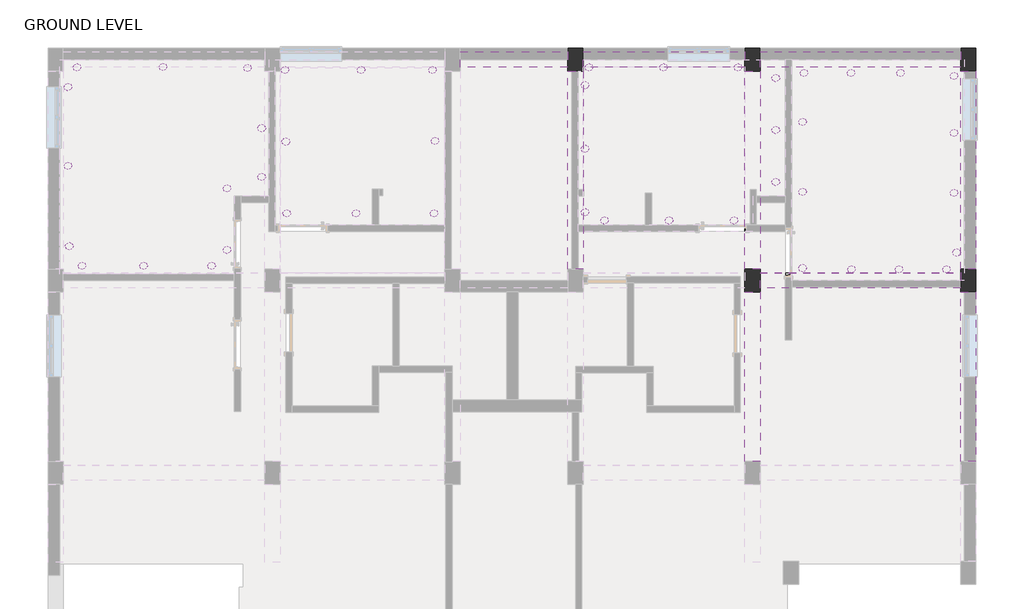
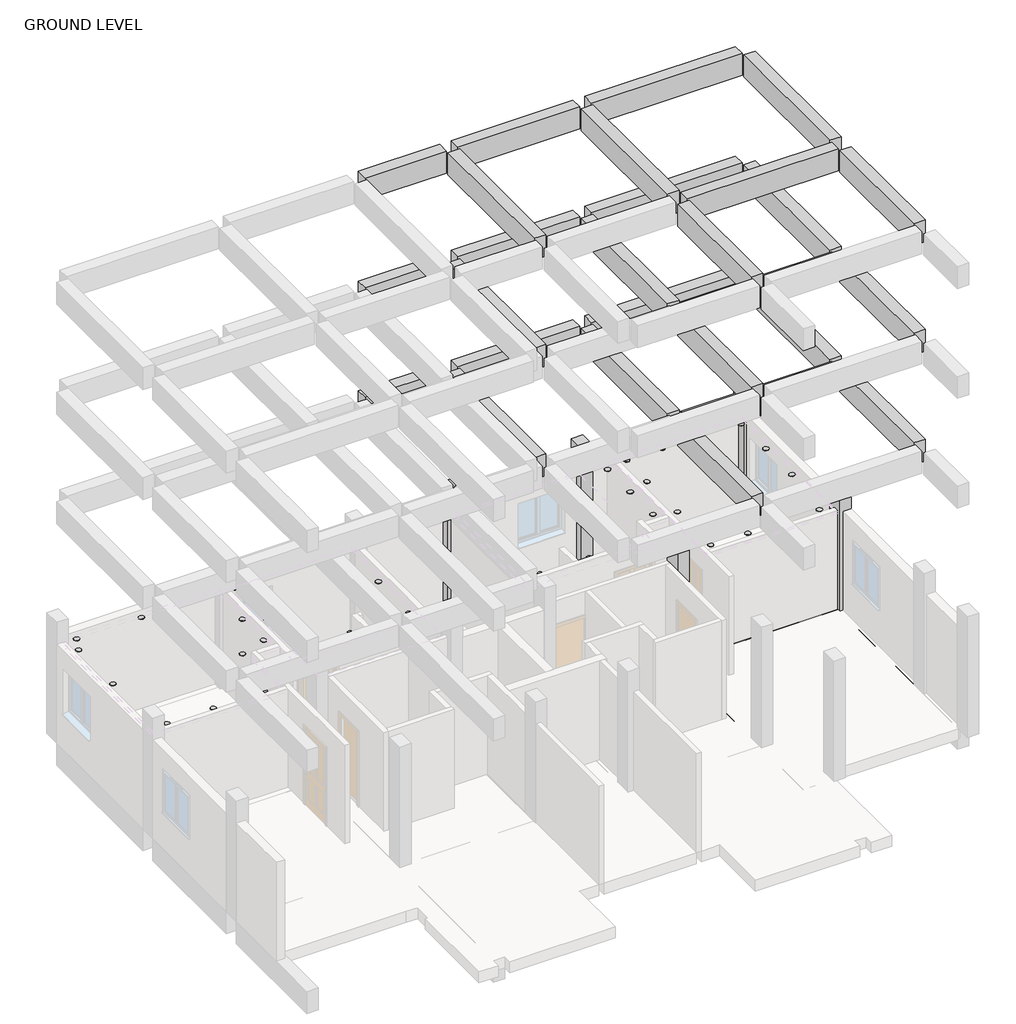
# One storey, part 5 of 5: 46 light fixtures, 36 beams, 5 columns.
"""IFC4 building model written with IfcOpenShell, lengths in millimetres."""

from ifc_helpers import new_model, si_unit, frame, origin, origin_with_axes, place, context, project, spatial, polyline, outline, extrude, faceted_brep, transform, mapped, element, save
from components import family2_family2_8c2629c1

model = new_model("IFC4")

# Units and contexts
model_context = context("Model", 3, world=origin())
ifc_project = project(units=[si_unit("LENGTHUNIT", "METRE", prefix="MILLI")], contexts=[model_context])

# Site, building, storey
site = spatial("IfcSite", under=ifc_project)
building = spatial("IfcBuilding", under=site)
storey = spatial("IfcBuildingStorey", under=building, Name="GROUND LEVEL", Elevation=0.0)

# Beams
placement = place(None, origin())
element("IfcBeam", 1, ObjectType="Concrete-Rectangular Beam : 12 x 24", at=placement, inside=storey, context=model_context, shape_type="SweptSolid", body=[
    extrude(outline(polyline([(1141.4824202, -1299.8061634), (1141.4824202, -1604.6061634), (-992.1175798, -1604.6061634), (-992.1175798, -1299.8061634), (1141.4824202, -1299.8061634)])), frame((0.0, 0.0, -609.6), z_axis=(0.0, 0.0, 1.0), x_axis=(1.0, 0.0, 0.0)), (0.0, 0.0, 1.0), 609.6),
])
element("IfcBeam", 2, ObjectType="Concrete-Rectangular Beam : 12 x 24", at=placement, inside=storey, context=model_context, shape_type="SweptSolid", body=[
    extrude(outline(polyline([(4646.6824202, -1299.8061634), (4646.6824202, -1604.6061634), (1446.2824202, -1604.6061634), (1446.2824202, -1299.8061634), (4646.6824202, -1299.8061634)])), frame((0.0, 0.0, -609.6), z_axis=(0.0, 0.0, 1.0), x_axis=(1.0, 0.0, 0.0)), (0.0, 0.0, 1.0), 609.6),
])
element("IfcBeam", 3, ObjectType="Concrete-Rectangular Beam : 12 x 24", at=placement, inside=storey, context=model_context, shape_type="SweptSolid", body=[
    extrude(outline(polyline([(8913.9345022, -1299.8061634), (8913.9345022, -1604.6061634), (4951.5345022, -1604.6061634), (4951.5345022, -1299.8061634), (8913.9345022, -1299.8061634)])), frame((0.0, 0.0, -609.6), z_axis=(0.0, 0.0, 1.0), x_axis=(1.0, 0.0, 0.0)), (0.0, 0.0, 1.0), 609.6),
])
element("IfcBeam", 4, ObjectType="Concrete-Rectangular Beam : 12 x 24", at=placement, inside=storey, context=model_context, shape_type="SweptSolid", body=[
    extrude(outline(polyline([(9218.6824202, -5600.6620333), (8913.8824202, -5600.6620333), (8913.8824202, -1680.8061634), (9218.6824202, -1680.8061634), (9218.6824202, -5600.6620333)])), frame((0.0, 0.0, -609.6), z_axis=(0.0, 0.0, 1.0), x_axis=(1.0, 0.0, 0.0)), (0.0, 0.0, 1.0), 609.6),
])
element("IfcBeam", 5, ObjectType="Concrete-Rectangular Beam : 12 x 24", at=placement, inside=storey, context=model_context, shape_type="SweptSolid", body=[
    extrude(outline(polyline([(9218.6824202, -9410.6620333), (8913.8824202, -9410.6620333), (8913.8824202, -6057.8620333), (9218.6824202, -6057.8620333), (9218.6824202, -9410.6620333)])), frame((0.0, 0.0, -609.6), z_axis=(0.0, 0.0, 1.0), x_axis=(1.0, 0.0, 0.0)), (0.0, 0.0, 1.0), 609.6),
])
element("IfcBeam", 6, ObjectType="Concrete-Rectangular Beam : 12 x 24", at=placement, inside=storey, context=model_context, shape_type="SweptSolid", body=[
    extrude(outline(polyline([(4951.4824202, -5981.6620333), (4951.4824202, -5676.8620333), (8913.8824202, -5676.8620333), (8913.8824202, -5981.6620333), (4951.4824202, -5981.6620333)])), frame((0.0, 0.0, -609.6), z_axis=(0.0, 0.0, 1.0), x_axis=(1.0, 0.0, 0.0)), (0.0, 0.0, 1.0), 609.6),
])
element("IfcBeam", 7, ObjectType="Concrete-Rectangular Beam : 12 x 24", at=placement, inside=storey, context=model_context, shape_type="SweptSolid", body=[
    extrude(outline(polyline([(1141.4824202, -1680.8061634), (1446.2824202, -1680.8061634), (1446.2824202, -5600.6620333), (1141.4824202, -5600.6620333), (1141.4824202, -1680.8061634)])), frame((0.0, 0.0, -609.6), z_axis=(0.0, 0.0, 1.0), x_axis=(1.0, 0.0, 0.0)), (0.0, 0.0, 1.0), 609.6),
])
element("IfcBeam", 8, ObjectType="Concrete-Rectangular Beam : 12 x 24", at=placement, inside=storey, context=model_context, shape_type="SweptSolid", body=[
    extrude(outline(polyline([(4951.4824202, -5600.6620333), (4646.6824202, -5600.6620333), (4646.6824202, -1680.8061634), (4951.4824202, -1680.8061634), (4951.4824202, -5600.6620333)])), frame((0.0, 0.0, -609.6), z_axis=(0.0, 0.0, 1.0), x_axis=(1.0, 0.0, 0.0)), (0.0, 0.0, 1.0), 609.6),
])
element("IfcBeam", 9, ObjectType="Concrete-Rectangular Beam : 12 x 24", at=placement, inside=storey, context=model_context, shape_type="SweptSolid", body=[
    extrude(outline(polyline([(4951.4824202, -9410.6620333), (4646.6824202, -9410.6620333), (4646.6824202, -6057.8620333), (4951.4824202, -6057.8620333), (4951.4824202, -9410.6620333)])), frame((0.0, 0.0, -609.6), z_axis=(0.0, 0.0, 1.0), x_axis=(1.0, 0.0, 0.0)), (0.0, 0.0, 1.0), 609.6),
])
element("IfcBeam", 10, ObjectType="Concrete-Rectangular Beam : 12 x 24", at=placement, inside=storey, context=model_context, shape_type="SweptSolid", body=[
    extrude(outline(polyline([(1141.4824202, -1299.8061634), (1141.4824202, -1604.6061634), (-992.1175798, -1604.6061634), (-992.1175798, -1299.8061634), (1141.4824202, -1299.8061634)])), frame((0.0, 0.0, 6096.0), z_axis=(0.0, 0.0, 1.0), x_axis=(1.0, 0.0, 0.0)), (0.0, 0.0, 1.0), 609.6),
])
element("IfcBeam", 11, ObjectType="Concrete-Rectangular Beam : 12 x 24", at=placement, inside=storey, context=model_context, shape_type="SweptSolid", body=[
    extrude(outline(polyline([(4646.6824202, -1299.8061634), (4646.6824202, -1604.6061634), (1446.2824202, -1604.6061634), (1446.2824202, -1299.8061634), (4646.6824202, -1299.8061634)])), frame((0.0, 0.0, 6096.0), z_axis=(0.0, 0.0, 1.0), x_axis=(1.0, 0.0, 0.0)), (0.0, 0.0, 1.0), 609.6),
])
element("IfcBeam", 12, ObjectType="Concrete-Rectangular Beam : 12 x 24", at=placement, inside=storey, context=model_context, shape_type="SweptSolid", body=[
    extrude(outline(polyline([(8913.9345022, -1299.8061634), (8913.9345022, -1604.6061634), (4951.5345022, -1604.6061634), (4951.5345022, -1299.8061634), (8913.9345022, -1299.8061634)])), frame((0.0, 0.0, 6096.0), z_axis=(0.0, 0.0, 1.0), x_axis=(1.0, 0.0, 0.0)), (0.0, 0.0, 1.0), 609.6),
])
element("IfcBeam", 13, ObjectType="Concrete-Rectangular Beam : 12 x 24", at=placement, inside=storey, context=model_context, shape_type="Brep", body=[
    faceted_brep([(8913.8824202, -5600.6620333, 6705.6), (9218.6824202, -5600.6620333, 6705.6), (9218.6824202, -1680.8061634, 6705.6), (8913.8824202, -1680.8061634, 6705.6), (8913.8824202, -5600.6620333, 6096.0), (8913.8824202, -5600.6620333, 6400.8), (8913.8824202, -1680.8061634, 6400.8), (8913.8824202, -1680.8061634, 6096.0), (9218.6824202, -5600.6620333, 6096.0), (9218.6824202, -1680.8061634, 6096.0), (9218.6824202, -5600.6620333, 6400.8), (9218.6824202, -1680.8061634, 6400.8)], [[[0, 1, 2, 3]], [[4, 5, 0, 3, 6, 7]], [[8, 4, 7, 9]], [[1, 10, 8, 9, 11, 2]], [[2, 11, 9, 7, 6, 3]], [[1, 0, 5, 4, 8, 10]]]),
])
element("IfcBeam", 14, ObjectType="Concrete-Rectangular Beam : 12 x 24", at=placement, inside=storey, context=model_context, shape_type="Brep", body=[
    faceted_brep([(8913.8824202, -9410.6620333, 6705.6), (9218.6824202, -9410.6620333, 6705.6), (9218.6824202, -6057.8620333, 6705.6), (8913.8824202, -6057.8620333, 6705.6), (8913.8824202, -9410.6620333, 6096.0), (8913.8824202, -9410.6620333, 6400.8), (8913.8824202, -6057.8620333, 6400.8), (8913.8824202, -6057.8620333, 6096.0), (9218.6824202, -9410.6620333, 6096.0), (9218.6824202, -6057.8620333, 6096.0), (9218.6824202, -9410.6620333, 6400.8), (9218.6824202, -6057.8620333, 6400.8)], [[[0, 1, 2, 3]], [[4, 5, 0, 3, 6, 7]], [[8, 4, 7, 9]], [[1, 10, 8, 9, 11, 2]], [[2, 11, 9, 7, 6, 3]], [[1, 0, 5, 4, 8, 10]]]),
])
element("IfcBeam", 15, ObjectType="Concrete-Rectangular Beam : 12 x 24", at=placement, inside=storey, context=model_context, shape_type="SweptSolid", body=[
    extrude(outline(polyline([(4951.4824202, -5981.6620333), (4951.4824202, -5676.8620333), (8913.8824202, -5676.8620333), (8913.8824202, -5981.6620333), (4951.4824202, -5981.6620333)])), frame((0.0, 0.0, 6096.0), z_axis=(0.0, 0.0, 1.0), x_axis=(1.0, 0.0, 0.0)), (0.0, 0.0, 1.0), 609.6),
])
element("IfcBeam", 16, ObjectType="Concrete-Rectangular Beam : 12 x 24", at=placement, inside=storey, context=model_context, shape_type="Brep", body=[
    faceted_brep([(1446.2824202, -1680.8061634, 6705.6), (1141.4824202, -1680.8061634, 6705.6), (1141.4824202, -5600.6620333, 6705.6), (1446.2824202, -5600.6620333, 6705.6), (1446.2824202, -1680.8061634, 6096.0), (1446.2824202, -1680.8061634, 6400.8), (1446.2824202, -5600.6620333, 6400.8), (1446.2824202, -5600.6620333, 6096.0), (1141.4824202, -1680.8061634, 6096.0), (1141.4824202, -5600.6620333, 6096.0), (1141.4824202, -1680.8061634, 6400.8), (1141.4824202, -5600.6620333, 6400.8)], [[[0, 1, 2, 3]], [[4, 5, 0, 3, 6, 7]], [[8, 4, 7, 9]], [[1, 10, 8, 9, 11, 2]], [[1, 0, 5, 4, 8, 10]], [[2, 11, 9, 7, 6, 3]]]),
])
element("IfcBeam", 17, ObjectType="Concrete-Rectangular Beam : 12 x 24", at=placement, inside=storey, context=model_context, shape_type="Brep", body=[
    faceted_brep([(4646.6824202, -5600.6620333, 6705.6), (4951.4824202, -5600.6620333, 6705.6), (4951.4824202, -1680.8061634, 6705.6), (4646.6824202, -1680.8061634, 6705.6), (4646.6824202, -5600.6620333, 6096.0), (4646.6824202, -5600.6620333, 6400.8), (4646.6824202, -1680.8061634, 6400.8), (4646.6824202, -1680.8061634, 6096.0), (4951.4824202, -5600.6620333, 6096.0), (4951.4824202, -1680.8061634, 6096.0), (4951.4824202, -5600.6620333, 6400.8), (4951.4824202, -1680.8061634, 6400.8)], [[[0, 1, 2, 3]], [[4, 5, 0, 3, 6, 7]], [[8, 4, 7, 9]], [[1, 10, 8, 9, 11, 2]], [[2, 11, 9, 7, 6, 3]], [[1, 0, 5, 4, 8, 10]]]),
])
element("IfcBeam", 18, ObjectType="Concrete-Rectangular Beam : 12 x 24", at=placement, inside=storey, context=model_context, shape_type="Brep", body=[
    faceted_brep([(4646.6824202, -9410.6620333, 6705.6), (4951.4824202, -9410.6620333, 6705.6), (4951.4824202, -6057.8620333, 6705.6), (4646.6824202, -6057.8620333, 6705.6), (4646.6824202, -9410.6620333, 6096.0), (4646.6824202, -9410.6620333, 6400.8), (4646.6824202, -6057.8620333, 6400.8), (4646.6824202, -6057.8620333, 6096.0), (4951.4824202, -9410.6620333, 6096.0), (4951.4824202, -6057.8620333, 6096.0), (4951.4824202, -9410.6620333, 6400.8), (4951.4824202, -6057.8620333, 6400.8)], [[[0, 1, 2, 3]], [[4, 5, 0, 3, 6, 7]], [[8, 4, 7, 9]], [[1, 10, 8, 9, 11, 2]], [[2, 11, 9, 7, 6, 3]], [[1, 0, 5, 4, 8, 10]]]),
])
element("IfcBeam", 19, ObjectType="Concrete-Rectangular Beam : 12 x 24", at=placement, inside=storey, context=model_context, shape_type="SweptSolid", body=[
    extrude(outline(polyline([(1141.4824202, -1299.8061634), (1141.4824202, -1604.6061634), (-992.1175798, -1604.6061634), (-992.1175798, -1299.8061634), (1141.4824202, -1299.8061634)])), frame((0.0, 0.0, 9144.0), z_axis=(0.0, 0.0, 1.0), x_axis=(1.0, 0.0, 0.0)), (0.0, 0.0, 1.0), 609.6),
])
element("IfcBeam", 20, ObjectType="Concrete-Rectangular Beam : 12 x 24", at=placement, inside=storey, context=model_context, shape_type="SweptSolid", body=[
    extrude(outline(polyline([(4646.6824202, -1299.8061634), (4646.6824202, -1604.6061634), (1446.2824202, -1604.6061634), (1446.2824202, -1299.8061634), (4646.6824202, -1299.8061634)])), frame((0.0, 0.0, 9144.0), z_axis=(0.0, 0.0, 1.0), x_axis=(1.0, 0.0, 0.0)), (0.0, 0.0, 1.0), 609.6),
])
element("IfcBeam", 21, ObjectType="Concrete-Rectangular Beam : 12 x 24", at=placement, inside=storey, context=model_context, shape_type="SweptSolid", body=[
    extrude(outline(polyline([(8913.9345022, -1299.8061634), (8913.9345022, -1604.6061634), (4951.5345022, -1604.6061634), (4951.5345022, -1299.8061634), (8913.9345022, -1299.8061634)])), frame((0.0, 0.0, 9144.0), z_axis=(0.0, 0.0, 1.0), x_axis=(1.0, 0.0, 0.0)), (0.0, 0.0, 1.0), 609.6),
])
element("IfcBeam", 22, ObjectType="Concrete-Rectangular Beam : 12 x 24", at=placement, inside=storey, context=model_context, shape_type="Brep", body=[
    faceted_brep([(8913.8824202, -5600.6620333, 9753.6), (9218.6824202, -5600.6620333, 9753.6), (9218.6824202, -1680.8061634, 9753.6), (8913.8824202, -1680.8061634, 9753.6), (8913.8824202, -5600.6620333, 9144.0), (8913.8824202, -5600.6620333, 9448.8), (8913.8824202, -1680.8061634, 9448.8), (8913.8824202, -1680.8061634, 9144.0), (9218.6824202, -5600.6620333, 9144.0), (9218.6824202, -1680.8061634, 9144.0), (9218.6824202, -5600.6620333, 9448.8), (9218.6824202, -1680.8061634, 9448.8)], [[[0, 1, 2, 3]], [[4, 5, 0, 3, 6, 7]], [[8, 4, 7, 9]], [[1, 10, 8, 9, 11, 2]], [[2, 11, 9, 7, 6, 3]], [[1, 0, 5, 4, 8, 10]]]),
])
element("IfcBeam", 23, ObjectType="Concrete-Rectangular Beam : 12 x 24", at=placement, inside=storey, context=model_context, shape_type="Brep", body=[
    faceted_brep([(8913.8824202, -9410.6620333, 9753.6), (9218.6824202, -9410.6620333, 9753.6), (9218.6824202, -6057.8620333, 9753.6), (8913.8824202, -6057.8620333, 9753.6), (8913.8824202, -9410.6620333, 9144.0), (8913.8824202, -9410.6620333, 9448.8), (8913.8824202, -6057.8620333, 9448.8), (8913.8824202, -6057.8620333, 9144.0), (9218.6824202, -9410.6620333, 9144.0), (9218.6824202, -6057.8620333, 9144.0), (9218.6824202, -9410.6620333, 9448.8), (9218.6824202, -6057.8620333, 9448.8)], [[[0, 1, 2, 3]], [[4, 5, 0, 3, 6, 7]], [[8, 4, 7, 9]], [[1, 10, 8, 9, 11, 2]], [[2, 11, 9, 7, 6, 3]], [[1, 0, 5, 4, 8, 10]]]),
])
element("IfcBeam", 24, ObjectType="Concrete-Rectangular Beam : 12 x 24", at=placement, inside=storey, context=model_context, shape_type="SweptSolid", body=[
    extrude(outline(polyline([(4951.4824202, -5981.6620333), (4951.4824202, -5676.8620333), (8913.8824202, -5676.8620333), (8913.8824202, -5981.6620333), (4951.4824202, -5981.6620333)])), frame((0.0, 0.0, 9144.0), z_axis=(0.0, 0.0, 1.0), x_axis=(1.0, 0.0, 0.0)), (0.0, 0.0, 1.0), 609.6),
])
element("IfcBeam", 25, ObjectType="Concrete-Rectangular Beam : 12 x 24", at=placement, inside=storey, context=model_context, shape_type="Brep", body=[
    faceted_brep([(1446.2824202, -1680.8061634, 9753.6), (1141.4824202, -1680.8061634, 9753.6), (1141.4824202, -5600.6620333, 9753.6), (1446.2824202, -5600.6620333, 9753.6), (1446.2824202, -1680.8061634, 9144.0), (1446.2824202, -1680.8061634, 9448.8), (1446.2824202, -5600.6620333, 9448.8), (1446.2824202, -5600.6620333, 9144.0), (1141.4824202, -1680.8061634, 9144.0), (1141.4824202, -5600.6620333, 9144.0), (1141.4824202, -1680.8061634, 9448.8), (1141.4824202, -5600.6620333, 9448.8)], [[[0, 1, 2, 3]], [[4, 5, 0, 3, 6, 7]], [[8, 4, 7, 9]], [[1, 10, 8, 9, 11, 2]], [[1, 0, 5, 4, 8, 10]], [[2, 11, 9, 7, 6, 3]]]),
])
element("IfcBeam", 26, ObjectType="Concrete-Rectangular Beam : 12 x 24", at=placement, inside=storey, context=model_context, shape_type="Brep", body=[
    faceted_brep([(4646.6824202, -5600.6620333, 9753.6), (4951.4824202, -5600.6620333, 9753.6), (4951.4824202, -1680.8061634, 9753.6), (4646.6824202, -1680.8061634, 9753.6), (4646.6824202, -5600.6620333, 9144.0), (4646.6824202, -5600.6620333, 9448.8), (4646.6824202, -1680.8061634, 9448.8), (4646.6824202, -1680.8061634, 9144.0), (4951.4824202, -5600.6620333, 9144.0), (4951.4824202, -1680.8061634, 9144.0), (4951.4824202, -5600.6620333, 9448.8), (4951.4824202, -1680.8061634, 9448.8)], [[[0, 1, 2, 3]], [[4, 5, 0, 3, 6, 7]], [[8, 4, 7, 9]], [[1, 10, 8, 9, 11, 2]], [[2, 11, 9, 7, 6, 3]], [[1, 0, 5, 4, 8, 10]]]),
])
element("IfcBeam", 27, ObjectType="Concrete-Rectangular Beam : 12 x 24", at=placement, inside=storey, context=model_context, shape_type="Brep", body=[
    faceted_brep([(4646.6824202, -9410.6620333, 9753.6), (4951.4824202, -9410.6620333, 9753.6), (4951.4824202, -6057.8620333, 9753.6), (4646.6824202, -6057.8620333, 9753.6), (4646.6824202, -9410.6620333, 9144.0), (4646.6824202, -9410.6620333, 9448.8), (4646.6824202, -6057.8620333, 9448.8), (4646.6824202, -6057.8620333, 9144.0), (4951.4824202, -9410.6620333, 9144.0), (4951.4824202, -6057.8620333, 9144.0), (4951.4824202, -9410.6620333, 9448.8), (4951.4824202, -6057.8620333, 9448.8)], [[[0, 1, 2, 3]], [[4, 5, 0, 3, 6, 7]], [[8, 4, 7, 9]], [[1, 10, 8, 9, 11, 2]], [[2, 11, 9, 7, 6, 3]], [[1, 0, 5, 4, 8, 10]]]),
])
element("IfcBeam", 28, ObjectType="Concrete-Rectangular Beam : 12 x 24", at=placement, inside=storey, context=model_context, shape_type="SweptSolid", body=[
    extrude(outline(polyline([(1141.4824202, -1299.8061634), (1141.4824202, -1604.6061634), (-992.1175798, -1604.6061634), (-992.1175798, -1299.8061634), (1141.4824202, -1299.8061634)])), frame((0.0, 0.0, 12192.0), z_axis=(0.0, 0.0, 1.0), x_axis=(1.0, 0.0, 0.0)), (0.0, 0.0, 1.0), 609.6),
])
element("IfcBeam", 29, ObjectType="Concrete-Rectangular Beam : 12 x 24", at=placement, inside=storey, context=model_context, shape_type="SweptSolid", body=[
    extrude(outline(polyline([(4646.6824202, -1299.8061634), (4646.6824202, -1604.6061634), (1446.2824202, -1604.6061634), (1446.2824202, -1299.8061634), (4646.6824202, -1299.8061634)])), frame((0.0, 0.0, 12192.0), z_axis=(0.0, 0.0, 1.0), x_axis=(1.0, 0.0, 0.0)), (0.0, 0.0, 1.0), 609.6),
])
element("IfcBeam", 30, ObjectType="Concrete-Rectangular Beam : 12 x 24", at=placement, inside=storey, context=model_context, shape_type="SweptSolid", body=[
    extrude(outline(polyline([(8913.9345022, -1299.8061634), (8913.9345022, -1604.6061634), (4951.5345022, -1604.6061634), (4951.5345022, -1299.8061634), (8913.9345022, -1299.8061634)])), frame((0.0, 0.0, 12192.0), z_axis=(0.0, 0.0, 1.0), x_axis=(1.0, 0.0, 0.0)), (0.0, 0.0, 1.0), 609.6),
])
element("IfcBeam", 31, ObjectType="Concrete-Rectangular Beam : 12 x 24", at=placement, inside=storey, context=model_context, shape_type="SweptSolid", body=[
    extrude(outline(polyline([(9218.6824202, -5600.6620333), (8913.8824202, -5600.6620333), (8913.8824202, -1680.8061634), (9218.6824202, -1680.8061634), (9218.6824202, -5600.6620333)])), frame((0.0, 0.0, 12192.0), z_axis=(0.0, 0.0, 1.0), x_axis=(1.0, 0.0, 0.0)), (0.0, 0.0, 1.0), 609.6),
])
element("IfcBeam", 32, ObjectType="Concrete-Rectangular Beam : 12 x 24", at=placement, inside=storey, context=model_context, shape_type="SweptSolid", body=[
    extrude(outline(polyline([(9218.6824202, -9410.6620333), (8913.8824202, -9410.6620333), (8913.8824202, -6057.8620333), (9218.6824202, -6057.8620333), (9218.6824202, -9410.6620333)])), frame((0.0, 0.0, 12192.0), z_axis=(0.0, 0.0, 1.0), x_axis=(1.0, 0.0, 0.0)), (0.0, 0.0, 1.0), 609.6),
])
element("IfcBeam", 33, ObjectType="Concrete-Rectangular Beam : 12 x 24", at=placement, inside=storey, context=model_context, shape_type="SweptSolid", body=[
    extrude(outline(polyline([(4951.4824202, -5981.6620333), (4951.4824202, -5676.8620333), (8913.8824202, -5676.8620333), (8913.8824202, -5981.6620333), (4951.4824202, -5981.6620333)])), frame((0.0, 0.0, 12192.0), z_axis=(0.0, 0.0, 1.0), x_axis=(1.0, 0.0, 0.0)), (0.0, 0.0, 1.0), 609.6),
])
element("IfcBeam", 34, ObjectType="Concrete-Rectangular Beam : 12 x 24", at=placement, inside=storey, context=model_context, shape_type="SweptSolid", body=[
    extrude(outline(polyline([(1141.4824202, -1680.8061634), (1446.2824202, -1680.8061634), (1446.2824202, -5600.6620333), (1141.4824202, -5600.6620333), (1141.4824202, -1680.8061634)])), frame((0.0, 0.0, 12192.0), z_axis=(0.0, 0.0, 1.0), x_axis=(1.0, 0.0, 0.0)), (0.0, 0.0, 1.0), 609.6),
])
element("IfcBeam", 35, ObjectType="Concrete-Rectangular Beam : 12 x 24", at=placement, inside=storey, context=model_context, shape_type="SweptSolid", body=[
    extrude(outline(polyline([(4951.4824202, -5600.6620333), (4646.6824202, -5600.6620333), (4646.6824202, -1680.8061634), (4951.4824202, -1680.8061634), (4951.4824202, -5600.6620333)])), frame((0.0, 0.0, 12192.0), z_axis=(0.0, 0.0, 1.0), x_axis=(1.0, 0.0, 0.0)), (0.0, 0.0, 1.0), 609.6),
])
element("IfcBeam", 36, ObjectType="Concrete-Rectangular Beam : 12 x 24", at=placement, inside=storey, context=model_context, shape_type="SweptSolid", body=[
    extrude(outline(polyline([(4951.4824202, -9410.6620333), (4646.6824202, -9410.6620333), (4646.6824202, -6057.8620333), (4951.4824202, -6057.8620333), (4951.4824202, -9410.6620333)])), frame((0.0, 0.0, 12192.0), z_axis=(0.0, 0.0, 1.0), x_axis=(1.0, 0.0, 0.0)), (0.0, 0.0, 1.0), 609.6),
])

# Columns
element("IfcColumn", 37, ObjectType="Concrete-Rectangular-Column : 1'6\" X 1' COLUMN", at=placement, inside=storey, context=model_context, shape_type="SweptSolid", body=[
    extrude(outline(polyline([(1446.2824202, -1223.6061634), (1446.2824202, -1680.8061634), (1141.4824202, -1680.8061634), (1141.4824202, -1223.6061634), (1446.2824202, -1223.6061634)])), origin_with_axes(), (0.0, 0.0, 1.0), 3352.8),
])
element("IfcColumn", 38, ObjectType="Concrete-Rectangular-Column : 1'6\" X 1' COLUMN", at=placement, inside=storey, context=model_context, shape_type="SweptSolid", body=[
    extrude(outline(polyline([(4951.4824202, -1223.6061634), (4951.4824202, -1680.8061634), (4646.6824202, -1680.8061634), (4646.6824202, -1223.6061634), (4951.4824202, -1223.6061634)])), origin_with_axes(), (0.0, 0.0, 1.0), 3352.8),
])
element("IfcColumn", 39, ObjectType="Concrete-Rectangular-Column : 1'6\" X 1' COLUMN", at=placement, inside=storey, context=model_context, shape_type="SweptSolid", body=[
    extrude(outline(polyline([(9218.6824202, -1223.6061634), (9218.6824202, -1680.8061634), (8913.8824202, -1680.8061634), (8913.8824202, -1223.6061634), (9218.6824202, -1223.6061634)])), origin_with_axes(), (0.0, 0.0, 1.0), 3352.8),
])
element("IfcColumn", 40, ObjectType="Concrete-Rectangular-Column : 1'6\" X 1' COLUMN", at=placement, inside=storey, context=model_context, shape_type="SweptSolid", body=[
    extrude(outline(polyline([(9218.6824202, -5600.6620333), (9218.6824202, -6057.8620333), (8913.8824202, -6057.8620333), (8913.8824202, -5600.6620333), (9218.6824202, -5600.6620333)])), origin_with_axes(), (0.0, 0.0, 1.0), 3352.8),
])
element("IfcColumn", 41, ObjectType="Concrete-Rectangular-Column : 1'6\" X 1' COLUMN", at=placement, inside=storey, context=model_context, shape_type="SweptSolid", body=[
    extrude(outline(polyline([(4951.4824202, -5600.6620333), (4951.4824202, -6057.8620333), (4646.6824202, -6057.8620333), (4646.6824202, -5600.6620333), (4951.4824202, -5600.6620333)])), origin_with_axes(), (0.0, 0.0, 1.0), 3352.8),
])

# Light fixtures
family2_family2_shape = family2_family2_8c2629c1(model_context)
element("IfcLightFixture", 42, ObjectType="Family2 : Family2", at=placement, inside=storey, context=model_context, shape_type="MappedRepresentation", body=[
    mapped(family2_family2_shape, transform((-4916.4175798, -3776.3061634, 101.6), x_axis=(1.0, 0.0, 0.0), y_axis=(0.0, 1.0, 0.0), z_axis=(0.0, 0.0, 1.0))),
])
element("IfcLightFixture", 43, ObjectType="Family2 : Family2", at=placement, inside=storey, context=model_context, shape_type="MappedRepresentation", body=[
    mapped(family2_family2_shape, transform((-4916.4175798, -2811.1061634, 101.6), x_axis=(1.0, 0.0, 0.0), y_axis=(0.0, 1.0, 0.0), z_axis=(0.0, 0.0, 1.0))),
])
element("IfcLightFixture", 44, ObjectType="Family2 : Family2", at=placement, inside=storey, context=model_context, shape_type="MappedRepresentation", body=[
    mapped(family2_family2_shape, transform((-5195.8175798, -1617.3061634, 101.6), x_axis=(1.0, 0.0, 0.0), y_axis=(0.0, 1.0, 0.0), z_axis=(0.0, 0.0, 1.0))),
])
element("IfcLightFixture", 45, ObjectType="Family2 : Family2", at=placement, inside=storey, context=model_context, shape_type="MappedRepresentation", body=[
    mapped(family2_family2_shape, transform((-8573.2786397, -1604.6061634, 101.6), x_axis=(1.0, 0.0, 0.0), y_axis=(0.0, 1.0, 0.0), z_axis=(0.0, 0.0, 1.0))),
])
element("IfcLightFixture", 46, ObjectType="Family2 : Family2", at=placement, inside=storey, context=model_context, shape_type="MappedRepresentation", body=[
    mapped(family2_family2_shape, transform((-6871.4786397, -1598.2561634, 101.6), x_axis=(1.0, 0.0, 0.0), y_axis=(0.0, 1.0, 0.0), z_axis=(0.0, 0.0, 1.0))),
])
element("IfcLightFixture", 47, ObjectType="Family2 : Family2", at=placement, inside=storey, context=model_context, shape_type="MappedRepresentation", body=[
    mapped(family2_family2_shape, transform((-8751.0786397, -1998.3061634, 101.6), x_axis=(1.0, 0.0, 0.0), y_axis=(0.0, 1.0, 0.0), z_axis=(0.0, 0.0, 1.0))),
])
element("IfcLightFixture", 48, ObjectType="Family2 : Family2", at=placement, inside=storey, context=model_context, shape_type="MappedRepresentation", body=[
    mapped(family2_family2_shape, transform((-8725.6786397, -5147.9061634, 101.6), x_axis=(1.0, 0.0, 0.0), y_axis=(0.0, 1.0, 0.0), z_axis=(0.0, 0.0, 1.0))),
])
element("IfcLightFixture", 49, ObjectType="Family2 : Family2", at=placement, inside=storey, context=model_context, shape_type="MappedRepresentation", body=[
    mapped(family2_family2_shape, transform((-8751.0786397, -3556.4104011, 101.6), x_axis=(1.0, 0.0, 0.0), y_axis=(0.0, 1.0, 0.0), z_axis=(0.0, 0.0, 1.0))),
])
element("IfcLightFixture", 50, ObjectType="Family2 : Family2", at=placement, inside=storey, context=model_context, shape_type="MappedRepresentation", body=[
    mapped(family2_family2_shape, transform((-8471.6786397, -5537.1620333, 101.6), x_axis=(1.0, 0.0, 0.0), y_axis=(0.0, 1.0, 0.0), z_axis=(0.0, 0.0, 1.0))),
])
element("IfcLightFixture", 51, ObjectType="Family2 : Family2", at=placement, inside=storey, context=model_context, shape_type="MappedRepresentation", body=[
    mapped(family2_family2_shape, transform((-5907.0175798, -5537.1620333, 101.6), x_axis=(1.0, 0.0, 0.0), y_axis=(0.0, 1.0, 0.0), z_axis=(0.0, 0.0, 1.0))),
])
element("IfcLightFixture", 52, ObjectType="Family2 : Family2", at=placement, inside=storey, context=model_context, shape_type="MappedRepresentation", body=[
    mapped(family2_family2_shape, transform((-7252.4786397, -5537.1620333, 101.6), x_axis=(1.0, 0.0, 0.0), y_axis=(0.0, 1.0, 0.0), z_axis=(0.0, 0.0, 1.0))),
])
element("IfcLightFixture", 53, ObjectType="Family2 : Family2", at=placement, inside=storey, context=model_context, shape_type="MappedRepresentation", body=[
    mapped(family2_family2_shape, transform((-5602.2175798, -5224.1061634, 101.6), x_axis=(1.0, 0.0, 0.0), y_axis=(0.0, 1.0, 0.0), z_axis=(0.0, 0.0, 1.0))),
])
element("IfcLightFixture", 54, ObjectType="Family2 : Family2", at=placement, inside=storey, context=model_context, shape_type="MappedRepresentation", body=[
    mapped(family2_family2_shape, transform((-5602.2175798, -4004.9061634, 101.6), x_axis=(1.0, 0.0, 0.0), y_axis=(0.0, 1.0, 0.0), z_axis=(0.0, 0.0, 1.0))),
])
element("IfcLightFixture", 55, ObjectType="Family2 : Family2", at=placement, inside=storey, context=model_context, shape_type="MappedRepresentation", body=[
    mapped(family2_family2_shape, transform((5815.0824202, -1718.9061634, 101.6), x_axis=(1.0, 0.0, 0.0), y_axis=(0.0, 1.0, 0.0), z_axis=(0.0, 0.0, 1.0))),
])
element("IfcLightFixture", 56, ObjectType="Family2 : Family2", at=placement, inside=storey, context=model_context, shape_type="MappedRepresentation", body=[
    mapped(family2_family2_shape, transform((8786.8824202, -1776.0561634, 101.6), x_axis=(1.0, 0.0, 0.0), y_axis=(0.0, 1.0, 0.0), z_axis=(0.0, 0.0, 1.0))),
])
element("IfcLightFixture", 57, ObjectType="Family2 : Family2", at=placement, inside=storey, context=model_context, shape_type="MappedRepresentation", body=[
    mapped(family2_family2_shape, transform((6746.4157535, -1718.9061634, 101.6), x_axis=(1.0, 0.0, 0.0), y_axis=(0.0, 1.0, 0.0), z_axis=(0.0, 0.0, 1.0))),
])
element("IfcLightFixture", 58, ObjectType="Family2 : Family2", at=placement, inside=storey, context=model_context, shape_type="MappedRepresentation", body=[
    mapped(family2_family2_shape, transform((7728.5490868, -1718.9061634, 101.6), x_axis=(1.0, 0.0, 0.0), y_axis=(0.0, 1.0, 0.0), z_axis=(0.0, 0.0, 1.0))),
])
element("IfcLightFixture", 59, ObjectType="Family2 : Family2", at=placement, inside=storey, context=model_context, shape_type="MappedRepresentation", body=[
    mapped(family2_family2_shape, transform((5789.6824202, -5582.2691591, 101.6), x_axis=(1.0, 0.0, 0.0), y_axis=(0.0, 1.0, 0.0), z_axis=(0.0, 0.0, 1.0))),
])
element("IfcLightFixture", 60, ObjectType="Family2 : Family2", at=placement, inside=storey, context=model_context, shape_type="MappedRepresentation", body=[
    mapped(family2_family2_shape, transform((8634.4824202, -5607.6691591, 101.6), x_axis=(1.0, 0.0, 0.0), y_axis=(0.0, 1.0, 0.0), z_axis=(0.0, 0.0, 1.0))),
])
element("IfcLightFixture", 61, ObjectType="Family2 : Family2", at=placement, inside=storey, context=model_context, shape_type="MappedRepresentation", body=[
    mapped(family2_family2_shape, transform((6754.8824202, -5607.6691591, 101.6), x_axis=(1.0, 0.0, 0.0), y_axis=(0.0, 1.0, 0.0), z_axis=(0.0, 0.0, 1.0))),
])
element("IfcLightFixture", 62, ObjectType="Family2 : Family2", at=placement, inside=storey, context=model_context, shape_type="MappedRepresentation", body=[
    mapped(family2_family2_shape, transform((7694.6824202, -5607.6691591, 101.6), x_axis=(1.0, 0.0, 0.0), y_axis=(0.0, 1.0, 0.0), z_axis=(0.0, 0.0, 1.0))),
])
element("IfcLightFixture", 63, ObjectType="Family2 : Family2", at=placement, inside=storey, context=model_context, shape_type="MappedRepresentation", body=[
    mapped(family2_family2_shape, transform((5789.6824202, -2686.6691591, 101.6), x_axis=(1.0, 0.0, 0.0), y_axis=(0.0, 1.0, 0.0), z_axis=(0.0, 0.0, 1.0))),
])
element("IfcLightFixture", 64, ObjectType="Family2 : Family2", at=placement, inside=storey, context=model_context, shape_type="MappedRepresentation", body=[
    mapped(family2_family2_shape, transform((5789.6824202, -4070.9691591, 101.6), x_axis=(1.0, 0.0, 0.0), y_axis=(0.0, 1.0, 0.0), z_axis=(0.0, 0.0, 1.0))),
])
element("IfcLightFixture", 65, ObjectType="Family2 : Family2", at=placement, inside=storey, context=model_context, shape_type="MappedRepresentation", body=[
    mapped(family2_family2_shape, transform((8837.6824202, -5274.9061634, 101.6), x_axis=(1.0, 0.0, 0.0), y_axis=(0.0, 1.0, 0.0), z_axis=(0.0, 0.0, 1.0))),
])
element("IfcLightFixture", 66, ObjectType="Family2 : Family2", at=placement, inside=storey, context=model_context, shape_type="MappedRepresentation", body=[
    mapped(family2_family2_shape, transform((8786.8824202, -2904.2394967, 101.6), x_axis=(1.0, 0.0, 0.0), y_axis=(0.0, 1.0, 0.0), z_axis=(0.0, 0.0, 1.0))),
])
element("IfcLightFixture", 67, ObjectType="Family2 : Family2", at=placement, inside=storey, context=model_context, shape_type="MappedRepresentation", body=[
    mapped(family2_family2_shape, transform((8786.8824202, -4089.57283, 101.6), x_axis=(1.0, 0.0, 0.0), y_axis=(0.0, 1.0, 0.0), z_axis=(0.0, 0.0, 1.0))),
])
element("IfcLightFixture", 68, ObjectType="Family2 : Family2", at=placement, inside=storey, context=model_context, shape_type="MappedRepresentation", body=[
    mapped(family2_family2_shape, transform((-4452.8675798, -1655.4061634, 101.6), x_axis=(1.0, 0.0, 0.0), y_axis=(0.0, 1.0, 0.0), z_axis=(0.0, 0.0, 1.0))),
])
element("IfcLightFixture", 69, ObjectType="Family2 : Family2", at=placement, inside=storey, context=model_context, shape_type="MappedRepresentation", body=[
    mapped(family2_family2_shape, transform((-1538.2175798, -1655.4061634, 101.6), x_axis=(1.0, 0.0, 0.0), y_axis=(0.0, 1.0, 0.0), z_axis=(0.0, 0.0, 1.0))),
])
element("IfcLightFixture", 70, ObjectType="Family2 : Family2", at=placement, inside=storey, context=model_context, shape_type="MappedRepresentation", body=[
    mapped(family2_family2_shape, transform((-2947.9175798, -1655.4061634, 101.6), x_axis=(1.0, 0.0, 0.0), y_axis=(0.0, 1.0, 0.0), z_axis=(0.0, 0.0, 1.0))),
])
element("IfcLightFixture", 71, ObjectType="Family2 : Family2", at=placement, inside=storey, context=model_context, shape_type="MappedRepresentation", body=[
    mapped(family2_family2_shape, transform((-4421.1175798, -4500.2061634, 101.6), x_axis=(1.0, 0.0, 0.0), y_axis=(0.0, 1.0, 0.0), z_axis=(0.0, 0.0, 1.0))),
])
element("IfcLightFixture", 72, ObjectType="Family2 : Family2", at=placement, inside=storey, context=model_context, shape_type="MappedRepresentation", body=[
    mapped(family2_family2_shape, transform((-4440.1675798, -3077.8061634, 101.6), x_axis=(1.0, 0.0, 0.0), y_axis=(0.0, 1.0, 0.0), z_axis=(0.0, 0.0, 1.0))),
])
element("IfcLightFixture", 73, ObjectType="Family2 : Family2", at=placement, inside=storey, context=model_context, shape_type="MappedRepresentation", body=[
    mapped(family2_family2_shape, transform((-1506.4675798, -4500.2061634, 101.6), x_axis=(1.0, 0.0, 0.0), y_axis=(0.0, 1.0, 0.0), z_axis=(0.0, 0.0, 1.0))),
])
element("IfcLightFixture", 74, ObjectType="Family2 : Family2", at=placement, inside=storey, context=model_context, shape_type="MappedRepresentation", body=[
    mapped(family2_family2_shape, transform((-3049.5175798, -4500.2061634, 101.6), x_axis=(1.0, 0.0, 0.0), y_axis=(0.0, 1.0, 0.0), z_axis=(0.0, 0.0, 1.0))),
])
element("IfcLightFixture", 75, ObjectType="Family2 : Family2", at=placement, inside=storey, context=model_context, shape_type="MappedRepresentation", body=[
    mapped(family2_family2_shape, transform((-1487.4175798, -3065.1061634, 101.6), x_axis=(1.0, 0.0, 0.0), y_axis=(0.0, 1.0, 0.0), z_axis=(0.0, 0.0, 1.0))),
])
element("IfcLightFixture", 76, ObjectType="Family2 : Family2", at=placement, inside=storey, context=model_context, shape_type="MappedRepresentation", body=[
    mapped(family2_family2_shape, transform((5256.2824202, -1820.5061634, 101.6), x_axis=(1.0, 0.0, 0.0), y_axis=(0.0, 1.0, 0.0), z_axis=(0.0, 0.0, 1.0))),
])
element("IfcLightFixture", 77, ObjectType="Family2 : Family2", at=placement, inside=storey, context=model_context, shape_type="MappedRepresentation", body=[
    mapped(family2_family2_shape, transform((5256.2824202, -3877.9061634, 101.6), x_axis=(1.0, 0.0, 0.0), y_axis=(0.0, 1.0, 0.0), z_axis=(0.0, 0.0, 1.0))),
])
element("IfcLightFixture", 78, ObjectType="Family2 : Family2", at=placement, inside=storey, context=model_context, shape_type="MappedRepresentation", body=[
    mapped(family2_family2_shape, transform((5256.2824202, -2849.2061634, 101.6), x_axis=(1.0, 0.0, 0.0), y_axis=(0.0, 1.0, 0.0), z_axis=(0.0, 0.0, 1.0))),
])
element("IfcLightFixture", 79, ObjectType="Family2 : Family2", at=placement, inside=storey, context=model_context, shape_type="MappedRepresentation", body=[
    mapped(family2_family2_shape, transform((1560.5824202, -1604.6061634, 101.6), x_axis=(1.0, 0.0, 0.0), y_axis=(0.0, 1.0, 0.0), z_axis=(0.0, 0.0, 1.0))),
])
element("IfcLightFixture", 80, ObjectType="Family2 : Family2", at=placement, inside=storey, context=model_context, shape_type="MappedRepresentation", body=[
    mapped(family2_family2_shape, transform((4506.9824202, -1604.6061634, 101.6), x_axis=(1.0, 0.0, 0.0), y_axis=(0.0, 1.0, 0.0), z_axis=(0.0, 0.0, 1.0))),
])
element("IfcLightFixture", 81, ObjectType="Family2 : Family2", at=placement, inside=storey, context=model_context, shape_type="MappedRepresentation", body=[
    mapped(family2_family2_shape, transform((3033.7824202, -1604.6061634, 101.6), x_axis=(1.0, 0.0, 0.0), y_axis=(0.0, 1.0, 0.0), z_axis=(0.0, 0.0, 1.0))),
])
element("IfcLightFixture", 82, ObjectType="Family2 : Family2", at=placement, inside=storey, context=model_context, shape_type="MappedRepresentation", body=[
    mapped(family2_family2_shape, transform((1484.3824202, -4474.8061634, 101.6), x_axis=(1.0, 0.0, 0.0), y_axis=(0.0, 1.0, 0.0), z_axis=(0.0, 0.0, 1.0))),
])
element("IfcLightFixture", 83, ObjectType="Family2 : Family2", at=placement, inside=storey, context=model_context, shape_type="MappedRepresentation", body=[
    mapped(family2_family2_shape, transform((1484.3824202, -1960.2061634, 101.6), x_axis=(1.0, 0.0, 0.0), y_axis=(0.0, 1.0, 0.0), z_axis=(0.0, 0.0, 1.0))),
])
element("IfcLightFixture", 84, ObjectType="Family2 : Family2", at=placement, inside=storey, context=model_context, shape_type="MappedRepresentation", body=[
    mapped(family2_family2_shape, transform((1484.3824202, -3217.5061634, 101.6), x_axis=(1.0, 0.0, 0.0), y_axis=(0.0, 1.0, 0.0), z_axis=(0.0, 0.0, 1.0))),
])
element("IfcLightFixture", 85, ObjectType="Family2 : Family2", at=placement, inside=storey, context=model_context, shape_type="MappedRepresentation", body=[
    mapped(family2_family2_shape, transform((4430.7824202, -4639.9061634, 101.6), x_axis=(1.0, 0.0, 0.0), y_axis=(0.0, 1.0, 0.0), z_axis=(0.0, 0.0, 1.0))),
])
element("IfcLightFixture", 86, ObjectType="Family2 : Family2", at=placement, inside=storey, context=model_context, shape_type="MappedRepresentation", body=[
    mapped(family2_family2_shape, transform((1865.3824202, -4639.9061634, 101.6), x_axis=(1.0, 0.0, 0.0), y_axis=(0.0, 1.0, 0.0), z_axis=(0.0, 0.0, 1.0))),
])
element("IfcLightFixture", 87, ObjectType="Family2 : Family2", at=placement, inside=storey, context=model_context, shape_type="MappedRepresentation", body=[
    mapped(family2_family2_shape, transform((3148.0824202, -4639.9061634, 101.6), x_axis=(1.0, 0.0, 0.0), y_axis=(0.0, 1.0, 0.0), z_axis=(0.0, 0.0, 1.0))),
])

save(model, "model.ifc")

# Revit data of these elements
# Type "Concrete-Rectangular Beam : 12 x 24"
#   Assembly Code = "B10"
#   Length [instance default] = 5' - 0"
#   b = 1' - 0"
#   h = 2' - 0"
#   Structural Material [instance default] = Concrete, Cast-in-Place gray
# Type "Concrete-Rectangular-Column : 1'6\" X 1' COLUMN"
#   Assembly Code = "B10"
#   b = 1' - 0"
#   h = 1' - 6"
#   Structural Material [instance default] = Concrete, Cast-in-Place gray
# Type "Family2 : Family2"
#   Wattage = 27 W
#   built-in parameter 1150110 = 1 (stored number, unit not read)
#   built-in parameter 1114217 = 1 (stored number, unit not read)
#   built-in parameter 1150109 = 1 (stored number, unit not read)
#   built-in parameter 1150113 = 1 (stored number, unit not read)
#   Lumens = 4010.63 lm
#   built-in parameter 1150115 = 1 (stored number, unit not read)
#   built-in parameter 1150105 = 319.156 (stored number, unit not read)
#   Light Source Symbol Size = 2' - 0"
#   built-in parameter 1150112 = 1 (stored number, unit not read)
#   built-in parameter 1150114 = 1 (stored number, unit not read)
#   built-in parameter 1150107 = 3000 (stored number, unit not read)
#   built-in parameter 1150106 = 3.19156 (stored number, unit not read)
#   built-in parameter 1150104 = 13.8 (stored number, unit not read)
#   built-in parameter 1114218 = 1 (stored number, unit not read)
#   built-in parameter 1150133 = 10 (stored number, unit not read)
#   Color Filter = 16777215
#   Dimming Lamp Color Temperature Shift = (empty or 0)
#   Default Elevation = 0
# Elements 1, 2, 3, 4, 5, 6, 7, 8, 9, 10, 11, 12, 13, 14, 15, 16, 17, 18, 19, 20, 21, 22, 23, 24, 25, 26, 27, 28, 29, 30, 31, 32, 33, 34, 35, 36 (IfcBeam, "Concrete-Rectangular Beam : 12 x 24")
#   Structural Material = WARM BEIGE COLOUR
#   Phase Created = New Construction
#   Materials on its faces: "WARM BEIGE COLOUR"
# Elements 37, 38, 39, 40, 41 (IfcColumn, "Concrete-Rectangular-Column : 1'6\" X 1' COLUMN")
#   Structural Material = WARM BEIGE COLOUR
#   Phase Created = New Construction
#   Materials on its faces: "WARM BEIGE COLOUR"
# Element 42 (IfcLightFixture, "Family2 : Family2")
#   Mark = "2"
#   Phase Created = New Construction
# Element 43 (IfcLightFixture, "Family2 : Family2")
#   Mark = "3"
#   Phase Created = New Construction
# Element 44 (IfcLightFixture, "Family2 : Family2")
#   Mark = "4"
#   Phase Created = New Construction
# Element 45 (IfcLightFixture, "Family2 : Family2")
#   Mark = "5"
#   Phase Created = New Construction
# Element 46 (IfcLightFixture, "Family2 : Family2")
#   Mark = "6"
#   Phase Created = New Construction
# Element 47 (IfcLightFixture, "Family2 : Family2")
#   Mark = "7"
#   Phase Created = New Construction
# Element 48 (IfcLightFixture, "Family2 : Family2")
#   Mark = "8"
#   Phase Created = New Construction
# Element 49 (IfcLightFixture, "Family2 : Family2")
#   Mark = "9"
#   Phase Created = New Construction
# Element 50 (IfcLightFixture, "Family2 : Family2")
#   Mark = "10"
#   Phase Created = New Construction
# Element 51 (IfcLightFixture, "Family2 : Family2")
#   Mark = "11"
#   Phase Created = New Construction
# Element 52 (IfcLightFixture, "Family2 : Family2")
#   Mark = "12"
#   Phase Created = New Construction
# Element 53 (IfcLightFixture, "Family2 : Family2")
#   Mark = "13"
#   Phase Created = New Construction
# Element 54 (IfcLightFixture, "Family2 : Family2")
#   Mark = "14"
#   Phase Created = New Construction
# Element 55 (IfcLightFixture, "Family2 : Family2")
#   Mark = "15"
#   Phase Created = New Construction
# Element 56 (IfcLightFixture, "Family2 : Family2")
#   Mark = "16"
#   Phase Created = New Construction
# Element 57 (IfcLightFixture, "Family2 : Family2")
#   Mark = "17"
#   Phase Created = New Construction
# Element 58 (IfcLightFixture, "Family2 : Family2")
#   Mark = "18"
#   Phase Created = New Construction
# Element 59 (IfcLightFixture, "Family2 : Family2")
#   Mark = "19"
#   Phase Created = New Construction
# Element 60 (IfcLightFixture, "Family2 : Family2")
#   Mark = "20"
#   Phase Created = New Construction
# Element 61 (IfcLightFixture, "Family2 : Family2")
#   Mark = "21"
#   Phase Created = New Construction
# Element 62 (IfcLightFixture, "Family2 : Family2")
#   Mark = "22"
#   Phase Created = New Construction
# Element 63 (IfcLightFixture, "Family2 : Family2")
#   Mark = "23"
#   Phase Created = New Construction
# Element 64 (IfcLightFixture, "Family2 : Family2")
#   Mark = "24"
#   Phase Created = New Construction
# Element 65 (IfcLightFixture, "Family2 : Family2")
#   Mark = "25"
#   Phase Created = New Construction
# Element 66 (IfcLightFixture, "Family2 : Family2")
#   Mark = "26"
#   Phase Created = New Construction
# Element 67 (IfcLightFixture, "Family2 : Family2")
#   Mark = "27"
#   Phase Created = New Construction
# Element 68 (IfcLightFixture, "Family2 : Family2")
#   Mark = "28"
#   Phase Created = New Construction
# Element 69 (IfcLightFixture, "Family2 : Family2")
#   Mark = "29"
#   Phase Created = New Construction
# Element 70 (IfcLightFixture, "Family2 : Family2")
#   Mark = "30"
#   Phase Created = New Construction
# Element 71 (IfcLightFixture, "Family2 : Family2")
#   Mark = "31"
#   Phase Created = New Construction
# Element 72 (IfcLightFixture, "Family2 : Family2")
#   Mark = "32"
#   Phase Created = New Construction
# Element 73 (IfcLightFixture, "Family2 : Family2")
#   Mark = "33"
#   Phase Created = New Construction
# Element 74 (IfcLightFixture, "Family2 : Family2")
#   Mark = "34"
#   Phase Created = New Construction
# Element 75 (IfcLightFixture, "Family2 : Family2")
#   Mark = "35"
#   Phase Created = New Construction
# Element 76 (IfcLightFixture, "Family2 : Family2")
#   Mark = "36"
#   Phase Created = New Construction
# Element 77 (IfcLightFixture, "Family2 : Family2")
#   Mark = "37"
#   Phase Created = New Construction
# Element 78 (IfcLightFixture, "Family2 : Family2")
#   Mark = "38"
#   Phase Created = New Construction
# Element 79 (IfcLightFixture, "Family2 : Family2")
#   Mark = "39"
#   Phase Created = New Construction
# Element 80 (IfcLightFixture, "Family2 : Family2")
#   Mark = "40"
#   Phase Created = New Construction
# Element 81 (IfcLightFixture, "Family2 : Family2")
#   Mark = "41"
#   Phase Created = New Construction
# Element 82 (IfcLightFixture, "Family2 : Family2")
#   Mark = "42"
#   Phase Created = New Construction
# Element 83 (IfcLightFixture, "Family2 : Family2")
#   Mark = "43"
#   Phase Created = New Construction
# Element 84 (IfcLightFixture, "Family2 : Family2")
#   Mark = "44"
#   Phase Created = New Construction
# Element 85 (IfcLightFixture, "Family2 : Family2")
#   Mark = "45"
#   Phase Created = New Construction
# Element 86 (IfcLightFixture, "Family2 : Family2")
#   Mark = "46"
#   Phase Created = New Construction
# Element 87 (IfcLightFixture, "Family2 : Family2")
#   Mark = "47"
#   Phase Created = New Construction
# Materials
#   "Concrete, Cast-in-Place gray": class "Concrete", colour RGB 192 192 192, transparency 0, Description = "Cast-in-place concrete", Cost = 0
#   "WARM BEIGE COLOUR": class "Generic", colour RGB 120 120 120, transparency 0, Cost = 0
